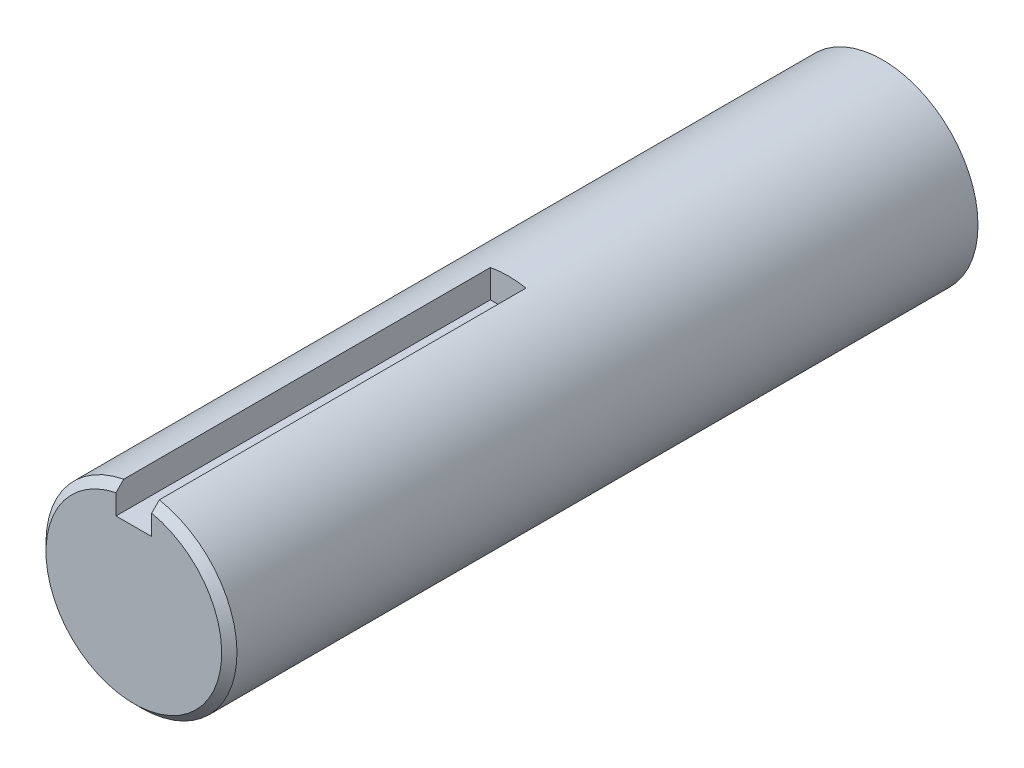
SolidWorks part; units mm, degrees
material "Plain Carbon Steel"
ref_plane "Front Plane" through (0, 0, 0) normal (0, 0, 1) x (1, 0, 0)
ref_plane "Top Plane" through (0, 0, 0) normal (0, 1, 0) x (1, 0, 0)
ref_plane "Right Plane" through (0, 0, 0) normal (1, 0, 0) x (0, 0, -1)
sketch "Shaft Profile Ø75" plane through (0, 0, 0) normal (0, 0, 1) x (1, 0, 0)
  circle A0 centre (0, 0) radius 37.5
  dimension "D1" = 75
extrude "Shaft Body Ø75x294" add sketch "Shaft Profile Ø75" along normal blind 294
sketch "Keyway Profile 14 wide" plane through (0, 0, 294) normal (0, 0, 1) x (1, 0, 0)
  line L0 (0, 0) -> (0, 55.631) construction
  line L2 (-7, 25.8409) -> (7, 25.8409)
  line L3 (-7, 25.8409) -> (-7, 36.8409)
  line L5 (7, 25.8409) -> (7, 36.8409)
  line L6 (-7, 25.8409) -> (7, 36.8409) construction
  line L7 (-7, 36.8409) -> (7, 25.8409) construction
  circle A0 centre (0, 0) radius 37.5 construction
  arc A1 (7, 36.8409) -> (-7, 36.8409) centre (0, 0) ccw
  point P3 (0, 31.3409)
  dimension "D1" = 14
  dimension "D2" = 11
extrude "Keyway Cut 14x147" cut sketch "Keyway Profile 14 wide" against normal blind 147
chamfer "End Chamfer 3x45°" distance 3 angle 45 1 edges at (0, -37.5, 294)
